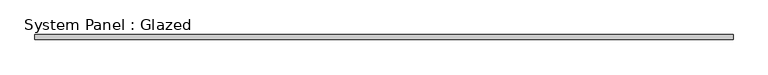
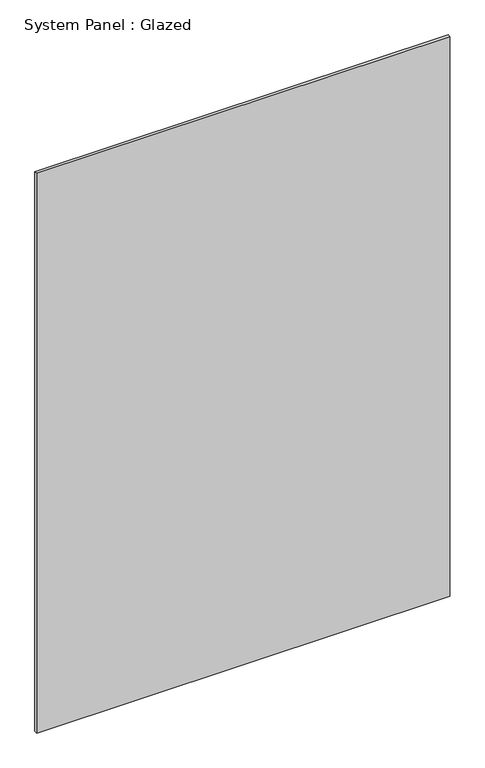
"""IFC4 building model written with IfcOpenShell, lengths in millimetres: plate geometry, System Panel : Glazed."""

from ifc_helpers import new_model, si_unit, origin, origin_with_axes, place, context, project, spatial, polyline, outline, extrude, source, transform, mapped, element, save


def system_panel_glazed_5cb243be(model_context):
    return source(origin(), model_context, "Body", "SweptSolid", [
        extrude(outline(polyline([(1765.1525428, 19.05), (-1765.1525428, 19.05), (-1765.1525428, 44.45), (1765.1525428, 44.45), (1765.1525428, 19.05)])), origin_with_axes(), (0.0, 0.0, 1.0), 5054.6),
    ])


if __name__ == "__main__":
    model = new_model("IFC4")
    model_context = context("Model", 3, world=origin())
    ifc_project = project(units=[si_unit("LENGTHUNIT", "METRE", prefix="MILLI")], contexts=[model_context])
    site = spatial("IfcSite", under=ifc_project)
    building = spatial("IfcBuilding", under=site)
    placement = place(None, origin())
    system_panel_glazed_shape = system_panel_glazed_5cb243be(model_context)
    element("IfcPlate", 1, ObjectType="System Panel : Glazed", at=placement, inside=building, context=model_context, shape_type="MappedRepresentation", body=[
        mapped(system_panel_glazed_shape, transform((0.0, 0.0, 0.0), x_axis=(1.0, 0.0, 0.0), y_axis=(0.0, 1.0, 0.0), z_axis=(0.0, 0.0, 1.0))),
    ])
    save(model, "model.ifc")

# Revit data of these elements
# Type "System Panel : Glazed"
#   Construction Type Id = "GSP4R"
#   Analytic Construction = "1/8 in Pilkington single glazing"
#   Visual Light Transmittance = 0.9
#   Solar Heat Gain Coefficient = 0.86
#   Heat Transfer Coefficient (U) = 1.18115 BTU/(h·ft²·°F)
# Element 1 (IfcPlate, "System Panel : Glazed")
#   Materials on its faces: "Glass"
# Materials
#   "Glass": class "Glass", colour RGB 0 128 192, transparency 0.75, Description = "Soda Lime Glass", Cost = 0
